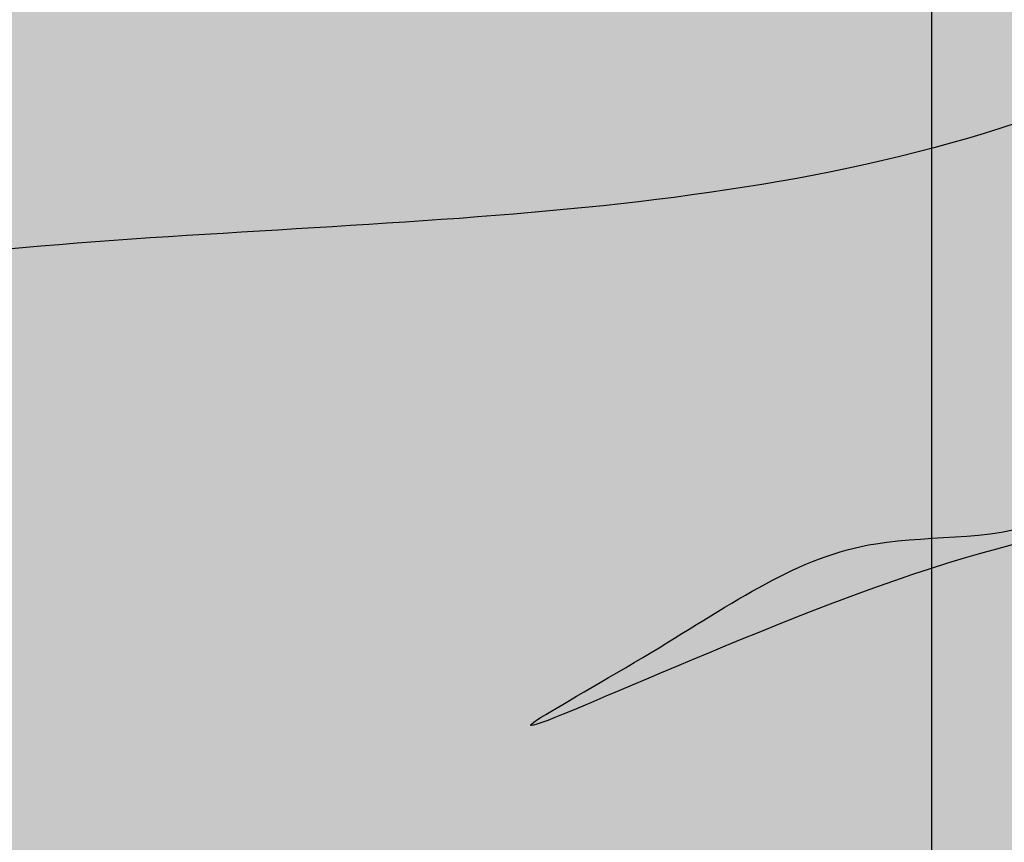
# Model space of a CAD drawing. Units: inches. Extents: x 1704 to 6393, y -157 to 1172.
# Tile 34 of 122: x 2529.29 to 2548.79, y 131.41 to 147.7. Entities that reach past the tile are written whole.
import ezdxf

# ---------------------------------------------------------------- set-up
doc = ezdxf.new("R2010")
doc.units = ezdxf.units.IN
doc.header["$MEASUREMENT"] = 0
for name, color, linetype, lineweight in [('A-ANNO-DIMS', 7, 'Continuous', 13), ('A-FURN', 8, 'Continuous', 18), ('estofado', 7, 'Continuous', 25)]:
    doc.layers.add(name, color=color, linetype=linetype, lineweight=lineweight)
doc.layers.add('A-FLOR-PATT', color=7, linetype='Continuous', lineweight=13, true_color=0xf2f2f2)
doc.styles.get("Standard").update_dxf_attribs({"font": 'arial.ttf'})
doc.dimstyles.get("Standard").update_dxf_attribs({"dimtxt": 6, "dimasz": 2, "dimexe": 0.18, "dimexo": 0.0625, "dimgap": 0.09, "dimtad": 0, "dimtih": 1, "dimtoh": 1, "dimdec": 1, "dimzin": 0, "dimdsep": 46, "dimlunit": 3, "dimtxsty": 'Standard', "dimblk": 'ARCHTICK', "dimcen": 0.09, "dimadec": 0, "dimazin": 0, "dimtfac": 1, "dimtdec": 1, "dimtofl": 0, "dimtmove": 0, "dimatfit": 3, "dimfxl": 1, "dimtolj": 1, "dimtzin": 0, "dimarcsym": 0})

# ---------------------------------------------------------------- blocks, each defined once
blk = doc.blocks.new('Cama Box Regencia LOLA')
at = {"layer": 'estofado', "ltscale": 0.2}
h = blk.add_hatch(color=256, dxfattribs=at)
h.dxf.hatch_style = 1
h.set_gradient(color1=(240, 232, 219), color2=(213, 190, 154), one_color=1, tint=0.7200000286102295, name='CURVED')
edge = h.paths.add_edge_path()
edge.add_spline(control_points=[(0.343533776195045, -0.8455058148597345), (0.2879313990920309, -0.8167160606696484), (0.2054770794474052, -0.7744470032542381), (0.0954193394759386, -0.7742416952675626), (-0.0885363502328574, -0.7276964167006668), (0.2428192566063672, -0.7672518992321216), (0.345087521536243, -0.8076697826234067), (0.3825206986321063, -0.8228555492498799)], knot_values=[0.0056315103357428, 0.0056315103357428, 0.0056315103357428, 0.0056315103357428, 0.1860138916206105, 0.2660015162584448, 0.3570871810327863, 0.5963901805690979, 0.739731738908988, 0.739731738908988, 0.739731738908988, 0.739731738908988], degree=3, periodic=0)
edge.add_spline(control_points=[(0.3825206986325611, -0.8228555492497662), (0.3974221570828149, -0.8135511441712424), (0.4121061736600496, -0.8037181558521524), (0.4266849906532571, -0.7937075488799225)], knot_values=[1.358237767273279, 1.358237767273279, 1.358237767273279, 1.358237767273279, 1.409915662372559, 1.409915662372559, 1.409915662372559, 1.409915662372559], degree=3, periodic=0)
edge.add_spline(control_points=[(0.4266849905698109, -0.7937075489369932), (0.3998777739682282, -0.7821381809783361), (0.3476761897024971, -0.7634757898491671), (0.2670618099601825, -0.7565375622627358), (0.0835725072796549, -0.7192994417154637), (0.288524529784695, -0.7446405493717521), (0.4247448861246994, -0.7759943071475277), (0.4449816270193879, -0.7810438091316882)], knot_values=[0.1043639306803623, 0.1043639306803623, 0.1043639306803623, 0.1043639306803623, 0.1896363068641149, 0.2696239315019491, 0.3607095962762907, 0.6000125958126024, 0.6446217338078729, 0.6446217338078729, 0.6446217338078729, 0.6446217338078729], degree=3, periodic=0)
edge.add_spline(control_points=[(0.4449816270197289, -0.7810438091316882), (0.5029779388527232, -0.7406836481117695), (0.5966687145296419, -0.6736247633211292), (0.7071737530245628, -0.6656573253703187), (0.7517012483331201, -0.6672238302253392)], knot_values=[1.43159032281798, 1.43159032281798, 1.43159032281798, 1.43159032281798, 1.63814180148235, 1.770695287284994, 1.770695287284994, 1.770695287284994, 1.770695287284994], degree=3, periodic=0)
edge.add_arc((0.7481853615017826, -0.767162003811734), 0.0999999999999888, 58.7920033978138, 87.98512997550938, ccw=False)
edge.add_line((0.8000000000000682, -0.6816328085782289), (0.8000000000000682, -0.154802362840428))
edge.add_line((0.8000000000000682, -0.154802362840428), (-0.7999999999999546, -0.154802362840428))
edge.add_line((-0.7999999999999546, -0.154802362840428), (-0.8000000000000682, -0.7409839258539819))
edge.add_spline(control_points=[(-0.799999999999841, -0.7409839258539251), (-0.7846451382113174, -0.74846387981205), (-0.7568940913494089, -0.7651582159765554), (-0.7559936909002545, -0.8096905380045313), (-0.7049413305308008, -0.8142555457367848), (-0.7013836936888538, -0.8139988647640733)], knot_values=[0.0122267587020837, 0.0122267587020837, 0.0122267587020837, 0.0122267587020837, 0.0594720782072034, 0.1062176618094138, 0.134458043575382, 0.134458043575382, 0.134458043575382, 0.134458043575382], degree=3, periodic=0)
edge.add_spline(control_points=[(-0.7013836936890812, -0.8139988647637892), (-0.6428309483887916, -0.8132695376718857), (-0.532520673001045, -0.8118955240036598), (-0.2390712668254764, -0.6717984706609172), (-0.3892411364554391, -0.7557901092520752), (-0.4591093260188473, -0.8070101468627512), (-0.5571511178645779, -0.795652750469742), (-0.608497950975675, -0.8409486634728295), (-0.6632498050151981, -0.8266781836207997), (-0.6991149398675134, -0.8254126024436914), (-0.719552182989446, -0.8246914287938125)], knot_values=[0, 0, 0, 0, 0.2187005959148062, 0.4120203559900679, 0.4786136596093368, 0.6046444033330721, 0.6969970394608519, 0.7456449795902803, 0.7925683322559657, 0.8547274388453192, 0.8547274388453192, 0.8547274388453192, 0.8547274388453192], degree=3, periodic=0)
edge.add_spline(control_points=[(-0.7195521829781911, -0.824691428792164), (-0.7293124663336812, -0.8248308281530967), (-0.7545977292818407, -0.8216412233076653), (-0.7742556984202338, -0.794819860189591), (-0.7939222919129634, -0.7820064600295497), (-0.799999999999841, -0.7800193173443404)], knot_values=[0.1564883932805935, 0.1564883932805935, 0.1564883932805935, 0.1564883932805935, 0.184397548386913, 0.2313764834161266, 0.2505984550882281, 0.2505984550882281, 0.2505984550882281, 0.2505984550882281], degree=3, periodic=0)
edge.add_line((-0.8000000000000682, -0.7800193173444541), (-0.7999999999999546, -0.8218505664627286))
edge.add_spline(control_points=[(-0.7999999999999546, -0.8218505664625013), (-0.7938082505512511, -0.8290217081292894), (-0.7673857405620766, -0.8512914803976059), (-0.7619109683460011, -0.8661369353891359), (-0.6555700939965164, -0.8510070218793543), (-0.7139793977868294, -0.8637526923380391), (-0.7379026254519659, -0.8623504601624176), (-0.7688129786438367, -0.8813042143888196), (-0.7854260296310259, -0.8561610219318254), (-0.7961930533253962, -0.8566031243811949), (-0.7999999999999546, -0.8573491405791173)], knot_values=[0.0595743221876141, 0.0595743221876141, 0.0595743221876141, 0.0595743221876141, 0.08075289116965, 0.1037414994169835, 0.1697200936249022, 0.1760361327243865, 0.2071371586311508, 0.2404744334261798, 0.2623408547027293, 0.2736604507987723, 0.2736604507987723, 0.2736604507987723, 0.2736604507987723], degree=3, periodic=0)
edge.add_line((-0.7999999999999546, -0.8573491405791173), (-0.8000000000000682, -0.9113562424721521))
edge.add_spline(control_points=[(-0.8000000000000682, -0.9113562424720385), (-0.7937204054647964, -0.9077594990848183), (-0.7710343135782978, -0.8978798065321029), (-0.7213062468074442, -0.9144666877443228), (-0.6268586829058905, -0.862430497409548), (-0.6896594748232019, -0.9045634991654196), (-0.7483442493064559, -0.9189273406958591), (-0.7835301183422417, -0.922920432793262), (-0.7896301351460125, -0.9477657000142585), (-0.7975786973822779, -0.955260590410262), (-0.8000000000001818, -0.9571831923294098)], knot_values=[0.0138560263374175, 0.0138560263374175, 0.0138560263374175, 0.0138560263374175, 0.0348737775836104, 0.0888666909546002, 0.1078792274429341, 0.1267378491223226, 0.1587140219647659, 0.1937574699451985, 0.2174867851300671, 0.2267221218327879, 0.2267221218327879, 0.2267221218327879, 0.2267221218327879], degree=3, periodic=0)
edge.add_line((-0.7999999999999546, -0.957183192329296), (-0.7999999999999546, -1.145824641594742))
edge.add_spline(control_points=[(-0.8000000000002955, -1.145824641594913), (-0.7271039467997298, -1.094596787649038), (-0.4885706936571524, -0.9465888221489535), (-0.0701640902225336, -0.9707493165000187), (0.237911901821235, -0.902164522332157), (0.3435337762145991, -0.845505814843193)], knot_values=[0.1168958193629841, 0.1168958193629841, 0.1168958193629841, 0.1168958193629841, 0.3797203297758731, 0.9577018633805092, 1.31379338443587, 1.31379338443587, 1.31379338443587, 1.31379338443587], degree=3, periodic=0)
h.paths.add_polyline_path([(-0.6766340706021765, -0.6101327540145576, -0.3575266660906883), (-0.7312746368313583, -0.6354535276154252, -0.3575266660894137), (-0.7059538632299791, -0.5808129613865844, -0.1647847126465284), (-0.7059538632300928, -0.2676124402649407, -0.3575266660890756), (-0.7312746368312446, -0.2129718740360431, -0.3575266660908716), (-0.6766340706020629, -0.2382926476369676, -0.0925607043966334), (-0.1295169377724505, -0.2382926476369107, -0.3575266660898965), (-0.0748763715433825, -0.2129718740360431, -0.3575266660894428), (-0.1001971451446479, -0.2676124402649407, -0.1647847126465285), (-0.1001971451445343, -0.5808129613865844, -0.3575266660890756), (-0.0748763715433825, -0.6354535276154821, -0.3575266660898962), (-0.1295169377724505, -0.6101327540146145, -0.0925607043966531)], flags=16)
h.paths.add_polyline_path([(0.0748763715433825, -0.6354535276157094, -0.3575266660910266), (0.1001971451446479, -0.5808129613865844, -0.1647847126465284), (0.1001971451445343, -0.2676124402649407, -0.3575266660890757), (0.0748763715433825, -0.2129718740360431, -0.3575266660898962), (0.1295169377724505, -0.2382926476369107, -0.0925607043966334), (0.6766340706020629, -0.2382926476369676, -0.3575266660908718), (0.7312746368312446, -0.2129718740360431, -0.3575266660894425), (0.7059538632299791, -0.2676124402649407, -0.1647847126465283), (0.7059538632300928, -0.5808129613865844, -0.3575266660890756), (0.7312746368312446, -0.6354535276154821, -0.3575266660908716), (0.6766340706020629, -0.6101327540145576, -0.0925607043966335), (0.1295169377724505, -0.6101327540146145, -0.3575266660906303)], flags=16)
h = blk.add_hatch(color=256, dxfattribs=at)
h.dxf.hatch_style = 1
h.set_gradient(color1=(206, 178, 131), color2=(227, 212, 186), one_color=1, tint=0.8100000023841857, name='CYLINDER')
edge = h.paths.add_edge_path()
edge.add_arc((0.7481853614966667, -0.7671620038115634), 0.0999999999999888, 342.0511336145294, 447.9851299725766)
edge.add_spline(control_points=[(0.7517012483331201, -0.6672238302253392), (0.7071737530245628, -0.6656573253703187), (0.5966687145298692, -0.6736247633211292), (0.5029779388527232, -0.7406836481117125), (0.4449816270195015, -0.7810438091316314)], knot_values=[1.431590322817835, 1.431590322817835, 1.431590322817835, 1.431590322817835, 1.564143808620479, 1.770695287284994, 1.770695287284994, 1.770695287284994, 1.770695287284994], degree=3, periodic=0)
edge.add_spline(control_points=[(0.4449816270195015, -0.7810438091316314), (0.4388957332065502, -0.7852790380018178), (0.4327996148541616, -0.7895089160493285), (0.4266849906533708, -0.7937075488798087)], knot_values=[1.409915662372814, 1.409915662372814, 1.409915662372814, 1.409915662372814, 1.431590322817835, 1.431590322817835, 1.431590322817835, 1.431590322817835], degree=3, periodic=0)
edge.add_spline(control_points=[(0.4266849906533708, -0.7937075488798087), (0.4121061736600496, -0.8037181558521524), (0.3974221570825875, -0.8135511441712991), (0.38252069863222, -0.8228555492498799)], knot_values=[1.358237767273037, 1.358237767273037, 1.358237767273037, 1.358237767273037, 1.409915662372815, 1.409915662372815, 1.409915662372815, 1.409915662372815], degree=3, periodic=0)
edge.add_line((0.3825206986330158, -0.8228555492493114), (0.343533776286904, -0.8455058148063584))
edge.add_spline(control_points=[(0.3435337761924302, -0.8455058148550165), (0.2379119018048641, -0.902164522335795), (-0.0701640902311738, -0.9707493164995071), (-0.4885706936571524, -0.9465888221488967), (-0.7271039467997298, -1.094596787649038), (-0.8000000000000682, -1.145824641594742)], knot_values=[0.1168958193630798, 0.1168958193630798, 0.1168958193630798, 0.1168958193630798, 0.472987340393773, 1.050968873998409, 1.313793384411202, 1.313793384411202, 1.313793384411202, 1.313793384411202], degree=3, periodic=0)
edge.add_spline(control_points=[(-0.8000000000000682, -1.145824641594742), (-0.8038896190357718, -1.14855807951244), (-0.8077744942224853, -1.151305646504738), (-0.8116551946761774, -1.154065647517199)], knot_values=[0.1028719158199011, 0.1028719158199011, 0.1028719158199011, 0.1028719158199011, 0.1168958193630799, 0.1168958193630799, 0.1168958193630799, 0.1168958193630799], degree=3, periodic=0)
edge.add_arc((-0.7536973518524519, -1.235557294053705), 0.1000000000000352, 125.4208969883762, 169.6981795679068)
edge.add_spline(control_points=[(-0.852085287466366, -1.217673946333093), (-0.8521399740518518, -1.217974812833915), (-0.8565649010855622, -1.242328483616745), (-0.8662697220019026, -1.297321141147904), (-0.8487158298532904, -1.34896742172242), (-0.8348745804664758, -1.381844109035796)], knot_values=[0.3128349436863077, 0.3128349436863077, 0.3128349436863077, 0.3128349436863077, 0.3137509534211996, 0.386958004641742, 0.4759027329026081, 0.4759027329026081, 0.4759027329026081, 0.4759027329026081], degree=3, periodic=0)
edge.add_spline(control_points=[(-0.8348745804664758, -1.38184410903591), (-0.8226532004149476, -1.367823298399059), (-0.8056354908857201, -1.352141651537124), (-0.7460155199962628, -1.32170802000337)], knot_values=[0.0062456970656236, 0.0062456970656236, 0.0062456970656236, 0.0062456970656236, 0.0554759259147193, 0.0554759259147193, 0.0554759259147193, 0.0554759259147193], degree=3, periodic=0)
edge.add_spline(control_points=[(-0.7460155200169539, -1.321708019985464), (-0.6188339616464873, -1.25080943574278), (-0.3488365122128698, -1.179158668568902), (0.0338148848931041, -1.279726484458706), (0.3977250465933366, -1.412092721352792), (0.6449024721503065, -1.106270719748692), (0.7873766543807506, -1.256744909425322), (0.8547271521993025, -1.327877176513538)], knot_values=[0.0991852523588446, 0.0991852523588446, 0.0991852523588446, 0.0991852523588446, 0.5236467270390676, 0.9270872950244264, 1.289918234564769, 1.564439021262726, 1.810554634340498, 1.810554634340498, 1.810554634340498, 1.810554634340498], degree=3, periodic=0)
edge.add_arc((0.5509678495186563, -1.223443291813453), 0.3212104454069235, 341.0267878798241, 383.7782184284114)
edge.add_arc((1.292676354991499, -0.9435407756057543), 0.4723459732861395, 162.0511336103901, 198.5657216587827, ccw=False)
h = blk.add_hatch(color=256, dxfattribs=at)
h.dxf.hatch_style = 1
h.set_gradient(color1=(240, 232, 219), color2=(137, 106, 57), one_color=1, tint=0.3799999952316284, name='CURVED')
edge = h.paths.add_edge_path()
edge.add_spline(control_points=[(-0.719552182989446, -0.8246914287938125), (-0.6991149398675134, -0.8254126024436914), (-0.6632498050151981, -0.8266781836207997), (-0.608497950975675, -0.8409486634728295), (-0.5571511178645779, -0.795652750469742), (-0.4591093260188473, -0.8070101468627512), (-0.3892411364554391, -0.7557901092520752), (-0.2390712668254764, -0.6717984706609172), (-0.532520673001045, -0.8118955240036598), (-0.6428309483887916, -0.8132695376718857), (-0.7013836936890812, -0.8139988647637892)], knot_values=[0, 0, 0, 0, 0.0621591065893537, 0.1090824592550391, 0.1577303993844675, 0.2500830355122473, 0.3761137792359825, 0.4427070828552515, 0.6360268429305131, 0.8547274388453192, 0.8547274388453192, 0.8547274388453192, 0.8547274388453192], degree=3, periodic=0)
edge.add_spline(control_points=[(-0.7013836936888538, -0.8139988647640733), (-0.7049413305308008, -0.8142555457367848), (-0.7559936909002545, -0.8096905380045313), (-0.7568940913494089, -0.7651582159765554), (-0.7846451382113174, -0.74846387981205), (-0.799999999999841, -0.7409839258539251)], knot_values=[0.0122267587020837, 0.0122267587020837, 0.0122267587020837, 0.0122267587020837, 0.0404671404680519, 0.0872127240702623, 0.134458043575382, 0.134458043575382, 0.134458043575382, 0.134458043575382], degree=3, periodic=0)
edge.add_spline(control_points=[(-0.799999999999841, -0.7409839258539251), (-0.798936373489596, -0.7431699116222604), (-0.7963938877088595, -0.7483952775559715), (-0.7912681985083055, -0.7566015403456845), (-0.7969680334608711, -0.7644035258254576), (-0.7929439183725436, -0.7707329795046576), (-0.7956241855360986, -0.7766169698310819), (-0.7985416092056994, -0.7788853679199974), (-0.7999999999999546, -0.7800193173443404)], knot_values=[0, 0, 0, 0, 0.0074537386837761, 0.0178173676883516, 0.0254983798788123, 0.0318742865004307, 0.0374248570653501, 0.0429729849735991, 0.0429729849735991, 0.0429729849735991, 0.0429729849735991], degree=3, periodic=0)
edge.add_spline(control_points=[(-0.799999999999841, -0.7800193173443404), (-0.7939222919129634, -0.7820064600295497), (-0.7742556984202338, -0.794819860189591), (-0.7545977292818407, -0.8216412233076653), (-0.7293124663336812, -0.8248308281530967), (-0.7195521829781911, -0.824691428792164)], knot_values=[0.1564883932805935, 0.1564883932805935, 0.1564883932805935, 0.1564883932805935, 0.175710364952695, 0.2226892999819086, 0.2505984550882281, 0.2505984550882281, 0.2505984550882281, 0.2505984550882281], degree=3, periodic=0)
h = blk.add_hatch(color=256, dxfattribs=at)
h.dxf.hatch_style = 1
h.set_gradient(color1=(240, 232, 219), color2=(137, 106, 57), one_color=1, tint=0.3799999952316284, name='CURVED')
edge = h.paths.add_edge_path()
edge.add_spline(control_points=[(0.3825206986321063, -0.8228555492498799), (0.345087521536243, -0.8076697826234067), (0.2428192566063672, -0.7672518992321216), (-0.0885363502328574, -0.7276964167006668), (0.0954193394759386, -0.7742416952675626), (0.2054770794474052, -0.7744470032542381), (0.2879313990920309, -0.8167160606696484), (0.343533776195045, -0.8455058148597345)], knot_values=[0.0056315103357428, 0.0056315103357428, 0.0056315103357428, 0.0056315103357428, 0.1489730686756328, 0.3882760682119444, 0.479361732986286, 0.5593493576241202, 0.739731738908988, 0.739731738908988, 0.739731738908988, 0.739731738908988], degree=3, periodic=0)
edge.add_line((0.343533776195045, -0.8455058148597913), (0.3825206986321063, -0.8228555492498799))
for points, knots in [([(-0.7013836936890812, -0.8139988647637892), (-0.6428309483887775, -0.8132695376718778), (-0.5325206730010296, -0.8118955240036225), (-0.2390712668254173, -0.6717984706608711), (-0.3892411364555083, -0.755790109252117), (-0.4591093260187714, -0.8070101468627889), (-0.5571511178644899, -0.795652750469717), (-0.6084979509757439, -0.8409486634728317), (-0.6632498050152652, -0.8266781836208043), (-0.6991149398675783, -0.8254126024437319), (-0.719552182989446, -0.8246914287938125)], [0, 0, 0, 0, 0.2187005959148062, 0.4120203559900679, 0.4786136596093368, 0.6046444033330721, 0.6969970394608519, 0.7456449795902803, 0.7925683322559657, 0.8547274388453192, 0.8547274388453192, 0.8547274388453192, 0.8547274388453192]), ([(-0.8116551946761774, -1.154065647517199), (-0.7350455857787211, -1.099579968801037), (-0.493473113061782, -0.9463057365681493), (-0.0701640902311738, -0.9707493164995071), (0.2379119018048641, -0.902164522335795), (0.3435337761924302, -0.8455058148550165)], [0.1028719158199011, 0.1028719158199011, 0.1028719158199011, 0.1028719158199011, 0.3797203297758731, 0.9577018633805092, 1.313793384411202, 1.313793384411202, 1.313793384411202, 1.313793384411202])]:
    blk.add_open_spline(points, degree=3, knots=knots, dxfattribs=at)
blk = doc.blocks.new('_ArchTick')
at = {"color": 0, "linetype": 'ByBlock', "const_width": 0.15}
blk.add_lwpolyline([(-0.5, -0.5), (0.5, 0.5)], dxfattribs=at)
blk = doc.blocks.new('*D93')
at = {"layer": 'A-ANNO-DIMS', "color": 0, "lineweight": -2, "transparency": 16777216}
for p, q in [((2605.286074000001, 895.2129740000005), (1829.697551000002, 895.2129740000003)), ((1829.877551000002, 895.2129740000003), (1829.877551000002, 495.8664119263302)), ((1829.877551000002, 90.2129739999999), (1829.877551000002, 489.5595360736699)), ((2605.286074000001, 90.21297400000003), (1829.697551000002, 90.2129739999999))]:
    blk.add_line(p, q, dxfattribs=at)
at = {"layer": 'Defpoints', "color": 0, "lineweight": -3, "transparency": 16777216}
for p in [(2605.348574000001, 895.2129740000005), (1829.877551000002, 90.2129739999999), (2605.348574000001, 90.21297400000003)]:
    blk.add_point(p, dxfattribs=at)
at = {"layer": 'A-ANNO-DIMS', "color": 0, "lineweight": -2, "transparency": 16777216, "xscale": 2, "yscale": 2, "zscale": 2}
for p, rotation in [((1829.877551000002, 895.2129740000003), 90), ((1829.877551000002, 90.2129739999999), 270)]:
    blk.add_blockref('_ArchTick', p, dxfattribs=dict(at, rotation=rotation))
at = {"layer": 'A-ANNO-DIMS', "color": 0, "transparency": 16777216, "insert": (1829.877551000001, 492.7129739999994), "char_height": 6, "attachment_point": 5}
blk.add_mtext('\\A1;805', dxfattribs=at)
blk = doc.blocks.new('*D105')
at = {"layer": 'A-ANNO-DIMS', "color": 0, "lineweight": -2, "transparency": 16777216}
for p, q in [((2451.737975, 615.150474), (2451.737975, -64.9670259999999)), ((2547.348574, 615.150474), (2547.348574, -64.9670259999999)), ((2451.737975, -64.787026), (2489.908936164393, -64.787026)), ((2547.348574, -64.787026), (2509.177612835607, -64.787026))]:
    blk.add_line(p, q, dxfattribs=at)
at = {"layer": 'Defpoints', "color": 0, "lineweight": -3, "transparency": 16777216}
for p in [(2451.737975, 615.212974), (2547.348574, 615.212974), (2547.348574, -64.787026)]:
    blk.add_point(p, dxfattribs=at)
at = {"layer": 'A-ANNO-DIMS', "color": 0, "lineweight": -2, "transparency": 16777216, "xscale": 2, "yscale": 2, "zscale": 2, "rotation": 180}
blk.add_blockref('_ArchTick', (2451.737975, -64.787026), dxfattribs=at)
at = {"layer": 'A-ANNO-DIMS', "color": 0, "lineweight": -2, "transparency": 16777216, "xscale": 2, "yscale": 2, "zscale": 2}
blk.add_blockref('_ArchTick', (2547.348574, -64.787026), dxfattribs=at)
at = {"layer": 'A-ANNO-DIMS', "color": 0, "transparency": 16777216, "insert": (2499.5432745, -64.787026), "char_height": 6, "attachment_point": 5}
blk.add_mtext('\\A1;95.61', dxfattribs=at)

msp = doc.modelspace()

# ---------------------------------------------------------------- hatches: boundary and pattern name
at = {"layer": 'A-FLOR-PATT', "transparency": 33554528}
h = msp.add_hatch(color=256, dxfattribs=at)
h.dxf.hatch_style = 1
h.paths.add_polyline_path([(2325.348574056059, 863.2129735309796), (2325.348574056059, 887.2129735309796), (2263.348574056059, 887.2129735309796), (2167.348574056059, 887.2129735309794), (2081.348574056061, 887.2129735309792), (2081.348574056061, 719.2129735309785), (2277.348574056059, 719.2129735309787), (2277.348574056059, 711.2129735309788), (2277.348574056059, 372.212973530979), (2349.348574056059, 372.212973530979), (2381.348574056059, 372.2129735309789), (2381.348574056059, 364.2129735309789), (2353.348574056059, 364.2129735309789), (2353.348574056059, 270.2129735309788), (2381.348574056059, 270.2129735309788), (2381.348574056059, 266.2129735309788), (2357.348574056059, 266.2129735309788), (2357.348574056059, 98.21297353097884), (2381.348574056059, 98.21297353097897), (2385.181056550604, 98.21297353097884), (2386.482186711948, 98.21297353097884), (2424.21496140017, 98.21297353097884), (2425.516091561514, 98.21297353097884), (2429.348574056059, 98.21297353097897), (2597.348574056059, 98.21297353097884), (2597.348574056059, 146.2129735309788), (2597.348574056059, 218.2129735309788), (2597.348574056059, 266.2129735309788), (2423.348574056059, 266.2129735309788), (2423.348574056059, 270.2129735309788), (2473.348574056059, 270.2129735309788), (2473.348574056059, 294.2129735309789), (2477.348574056059, 294.2129735309789), (2477.348574056059, 270.2129735309788), (2547.348574056059, 270.2129735309788), (2547.348574056059, 364.2129735309788), (2477.348574056059, 364.2129735309788), (2477.348574056059, 318.2129735309788), (2473.348574056059, 318.2129735309787), (2473.348574056059, 364.2129735309789), (2423.348574056059, 364.2129735309788), (2423.348574056059, 372.2129735309788), (2469.348574056059, 372.2129735309788), (2469.348574056059, 459.2129735309789), (2469.348574056059, 538.2129735309788), (2350.348574056059, 538.2129735309788), (2350.348574056059, 565.7129735309788), (2358.348574056059, 565.7129735309788), (2358.348574056059, 545.2129735309788), (2420.348574056059, 545.2129735309788), (2420.348574056059, 610.2129735309788), (2358.348574056059, 610.2129735309788), (2358.348574056059, 589.7129735309788), (2350.348574056059, 589.7129735309788), (2350.348574056059, 615.2129735309788), (2425.348574056059, 615.2129735309788), (2425.348574056059, 607.2129735309788), (2425.348574056059, 546.2129735309788), (2469.348574056059, 546.2129735309788), (2514.34857405606, 546.212973530979), (2514.34857405606, 607.2129735309788), (2449.348574056059, 607.2129735309788), (2449.348574056059, 615.2129735309788), (2451.737974987759, 615.2129735309788), (2451.737974987759, 659.2129735309788), (2427.737974987759, 659.2129735309788), (2427.737974987759, 665.2129735309788), (2367.737974987758, 665.2129735309788), (2367.737974987758, 667.2129735309788), (2367.737974987758, 711.2129735309788), (2325.348574056059, 711.2129735309788), (2325.348574056059, 719.2129735309785), (2325.348574056059, 755.2129735309787), (2325.348574056059, 763.2129735309788)])
h.paths.add_polyline_path([(2233.85817000392, 822.532660166629, -0.1872470486944155), (2233.85817000392, 809.1396667958562), (2231.697030374885, 808.8044951349628, 0.0848927708004382), (2233.130501812631, 814.4858417746204), (2230.423974436808, 814.4858417746204, -0.1042581087707907), (2228.553363812687, 808.3129425443484), (2217.750790159711, 807.1555239386723, -0.2222222222222219), (2217.750790159711, 824.5168030238124), (2228.553363812687, 823.3593844181363, -0.1042581087707933), (2230.423974436808, 817.1864851878643), (2233.130501812631, 817.1864851878643, 0.08489277080044), (2231.697030374885, 822.8678318275219)], flags=16)
h.paths.add_polyline_path([(2213.621360876743, 833.1974425663823), (2213.621360876743, 798.4748843961024), (2156.047684459484, 798.4748843961034), (2156.047684459485, 833.1974425663813)], flags=16)
h.paths.add_polyline_path([(2203.931929661768, 848.0987249710489), (2205.089348267444, 837.2961513180724, -0.2222222222222264), (2187.728069182304, 837.2961513180724), (2188.88548778798, 848.0987249710485, -0.104258108770792), (2195.058387018252, 849.9693355951691), (2195.058387018252, 852.6758629709927, 0.084892770800438), (2189.377040378595, 851.2423915332469), (2189.712212039488, 853.4035311622828, -0.1872470486944166), (2203.105205410261, 853.4035311622828), (2203.440377071154, 851.2423915332469, 0.084892770800438), (2197.759030431496, 852.6758629709927), (2197.759030431496, 849.9693355951691, -0.1042581087707896)], flags=16)
h.paths.add_polyline_path([(2181.940976153924, 837.2961513180726, -0.2222222222222323), (2164.579697068783, 837.2961513180724), (2165.73711567446, 848.0987249710487, -0.1042581087707905), (2171.910014904732, 849.9693355951691), (2171.910014904732, 852.6758629709927, 0.0848927708004445), (2166.228668265074, 851.2423915332469), (2166.563839925967, 853.403531162283, -0.1872470486944096), (2179.95683329674, 853.4035311622828), (2180.292004957633, 851.2423915332465, 0.0848927708004458), (2174.610658317976, 852.6758629709927), (2174.610658317976, 849.9693355951691, -0.104258108770801), (2180.783557548248, 848.0987249710482)], flags=16)
h.paths.add_polyline_path([(2205.089348267444, 794.376175644412), (2203.931929661768, 783.5736019914364, -0.1042581087707934), (2197.759030431496, 781.7029913673155), (2197.759030431496, 778.9964639914921, 0.084892770800439), (2203.440377071154, 780.4299354292382), (2203.105205410261, 778.2687958002022, -0.1872470486944172), (2189.712212039488, 778.2687958002018), (2189.377040378595, 780.4299354292377, 0.0848927708004369), (2195.058387018252, 778.9964639914919), (2195.058387018252, 781.7029913673153, -0.1042581087707904), (2188.88548778798, 783.5736019914358), (2187.728069182304, 794.3761756444126, -0.2222222222222231)], flags=16)
h.paths.add_polyline_path([(2181.940976153924, 794.376175644412), (2180.783557548248, 783.5736019914364, -0.1042581087708008), (2174.610658317976, 781.7029913673153), (2174.610658317976, 778.9964639914921, 0.0848927708004458), (2180.292004957633, 780.4299354292382), (2179.95683329674, 778.268795800202, -0.1872470486944096), (2166.563839925967, 778.2687958002018), (2166.228668265074, 780.4299354292378, 0.0848927708004446), (2171.910014904732, 778.9964639914919), (2171.910014904732, 781.7029913673153, -0.1042581087707904), (2165.73711567446, 783.5736019914358), (2164.579697068783, 794.3761756444123, -0.2222222222222294)], flags=16)
h.paths.add_polyline_path([(2151.918255176517, 807.1555239386723), (2141.115681523541, 808.3129425443484, -0.1042581087707911), (2139.24507089942, 814.4858417746204), (2136.538543523597, 814.4858417746204, 0.08489277080044), (2137.972014961343, 808.8044951349626), (2135.810875332307, 809.1396667958562, -0.1872470486944109), (2135.810875332307, 822.5326601666285), (2137.972014961343, 822.8678318275221, 0.0848927708004416), (2136.538543523597, 817.1864851878643), (2139.24507089942, 817.1864851878643, -0.104258108770793), (2141.115681523541, 823.3593844181363), (2151.918255176517, 824.5168030238124, -0.2222222222222205)], flags=16)
h.paths.add_polyline_path([(2357.868011454448, 363.4102250290031), (2358.813881560335, 363.4102250290031, 0.7537604849588476)], flags=16)
h.paths.add_polyline_path([(2372.241054283868, 363.1167008961685), (2372.248110816919, 363.1167008961685), (2372.248110816919, 363.3425764997267), (2371.30224071103, 363.3425764997267), (2371.30224071103, 363.1392706554335, -1.360391292333951)], flags=16)
h.paths.add_polyline_path([(2371.309297244092, 272.7157694655011), (2371.30224071103, 272.7157694655011), (2371.30224071103, 272.4898938619428), (2372.248110816919, 272.4898938619428), (2372.248110816919, 272.6931997062759, -1.360391292393621)], flags=16)
h.paths.add_polyline_path([(2357.875067987504, 272.7157694655011), (2357.868011454452, 272.7157694655011), (2357.868011454452, 272.4898938619428), (2358.813881560341, 272.4898938619428), (2358.813881560341, 272.6931997062361, -1.360391292333948)], flags=16)
h.paths.add_polyline_path([(2353.768696905258, 363.0736921025416), (2376.347425366111, 363.0736921025416), (2376.347425366111, 272.7587782591281), (2353.768696905258, 272.7587782591281)], flags=16)
h.paths.add_polyline_path([(2354.772195947961, 362.0701930598379), (2375.343926323407, 362.0701930598379), (2375.343926323407, 273.7622773018316), (2354.772195947961, 273.7622773018318)], flags=0)
h.paths.add_polyline_path([(2357.868011454452, 363.3425764997267), (2358.813881560341, 363.3425764997266), (2358.813881560341, 363.1167008961684), (2357.868011454452, 363.1167008961684)], flags=16)
h.paths.add_polyline_path([(2359.287941640134, 359.1843485433627), (2359.287941640134, 360.0631949744305), (2370.828180631237, 360.0631949744362), (2370.828180631237, 359.1843485433769), (2374.332057422314, 359.1843485433812), (2374.332057422312, 358.4635369582513), (2372.835178716611, 358.4635369582524), (2372.835178716611, 357.5410357047662), (2374.332057422314, 357.5410357047678), (2374.332057422312, 356.8202241196381), (2372.835178716611, 356.820224119639), (2372.835178716611, 355.897722866153), (2374.332057422314, 355.8977228661546), (2374.332057422312, 355.1769112810248), (2372.835178716611, 355.1769112810259), (2372.835178716611, 354.2544100275397), (2374.332057422334, 354.2544100275415), (2374.332057422331, 353.5335984424117), (2372.835178716631, 353.5335984424126), (2372.835178716631, 352.6110971889265), (2374.332057422334, 352.6110971889282), (2374.332057422331, 351.8902856037984), (2372.835178716631, 351.8902856037993), (2372.835178716631, 350.9677843503132), (2374.332057422334, 350.967784350315), (2374.332057422331, 350.2469727651852), (2372.835178716631, 350.2469727651861), (2372.835178716631, 349.3244715117), (2374.332057422334, 349.3244715117017), (2374.332057422331, 348.603659926572), (2372.835178716631, 348.6036599265729), (2372.835178716631, 347.6811586730868), (2374.332057422334, 347.6811586730886), (2374.332057422331, 346.9603470879587), (2372.835178716631, 346.9603470879598), (2372.835178716631, 346.0378458344735), (2374.332057422334, 346.0378458344753), (2374.332057422331, 345.3170342493456), (2372.835178716631, 345.3170342493465), (2372.835178716631, 344.3945329958605), (2374.332057422334, 344.3945329958621), (2374.332057422331, 343.6737214107324), (2372.835178716631, 343.6737214107334), (2372.835178716631, 342.751220157247), (2374.332057422334, 342.7512201572489), (2374.332057422331, 342.0304085721191), (2372.835178716631, 342.03040857212), (2372.835178716631, 341.1079073186338), (2374.332057422334, 341.1079073186356), (2374.332057422331, 340.3870957335057), (2372.835178716631, 340.3870957335066), (2372.835178716631, 339.4645944800207), (2374.332057422334, 339.4645944800223), (2374.332057422331, 338.7437828948924), (2372.835178716648, 338.7437828948933), (2372.835178716648, 337.8212816414076), (2374.332057422334, 337.8212816414093), (2374.332057422331, 337.1004700562794), (2372.835178716648, 337.1004700562803), (2372.835178716648, 336.1779688027942), (2374.332057422334, 336.1779688027961), (2374.332057422331, 335.4571572176662), (2372.835178716648, 335.4571572176673), (2372.835178716648, 334.5346559641809), (2374.332057422334, 334.5346559641828), (2374.332057422331, 333.8138443790529), (2372.835178716648, 333.8138443790539), (2372.835178716648, 332.8913431255679), (2374.332057422334, 332.8913431255696), (2374.332057422331, 332.1705315404397), (2372.835178716648, 332.1705315404406), (2372.835178716648, 331.2480302869545), (2374.332057422334, 331.2480302869563), (2374.332057422331, 330.5272187018265), (2372.835178716648, 330.5272187018273), (2372.835178716648, 329.6047174483413), (2374.332057422334, 329.6047174483431), (2374.332057422331, 328.8839058632133), (2372.835178716648, 328.8839058632143), (2372.835178716648, 327.9614046097282), (2374.332057422334, 327.9614046097298), (2374.332057422331, 327.2405930246), (2372.835178716648, 327.2405930246009), (2372.835178716648, 326.3180917711149), (2374.332057422334, 326.3180917711167), (2374.332057422331, 325.5972801859869), (2372.835178716648, 325.5972801859877), (2372.835178716648, 324.6747789325016), (2374.332057422334, 324.6747789325034), (2374.332057422331, 323.9539673473736), (2372.835178716648, 323.9539673473746), (2372.835178716648, 323.0314660938884), (2374.332057422334, 323.0314660938901), (2374.332057422331, 322.3106545087603), (2372.835178716648, 322.3106545087613), (2372.835178716648, 321.3881532552753), (2374.332057422334, 321.388153255277), (2374.332057422331, 320.6673416701471), (2372.835178716648, 320.6673416701481), (2372.835178716648, 319.7448404166621), (2374.332057422334, 319.7448404166638), (2374.332057422331, 319.0240288315339), (2372.835178716648, 319.0240288315348), (2372.835178716648, 318.1015275780487), (2374.332057422334, 318.1015275780504), (2374.332057422331, 317.3807159929205), (2372.835178716648, 317.3807159929214), (2372.835178716648, 316.4582147394357), (2374.332057422334, 316.4582147394373), (2374.332057422331, 315.7374031543073), (2372.835178716648, 315.7374031543084), (2372.835178716648, 314.8149019008223), (2374.332057422334, 314.8149019008241), (2374.332057422331, 314.0940903156943), (2372.835178716648, 314.0940903156952), (2372.835178716648, 313.171589062209), (2374.332057422334, 313.1715890622108), (2374.332057422331, 312.450777477081), (2372.835178716648, 312.4507774770819), (2372.835178716648, 311.5282762235959), (2374.332057422334, 311.5282762235977), (2374.332057422331, 310.8074646384678), (2372.835178716648, 310.8074646384687), (2372.835178716648, 309.8849633849827), (2374.332057422334, 309.8849633849844), (2374.332057422331, 309.1641517998546), (2372.835178716648, 309.1641517998555), (2372.835178716648, 308.2416505463693), (2374.332057422334, 308.2416505463712), (2374.332057422331, 307.5208389612412), (2372.835178716648, 307.5208389612421), (2372.835178716648, 306.5983377077562), (2374.332057422334, 306.598337707758), (2374.332057422331, 305.8775261226281), (2372.835178716648, 305.8775261226289), (2372.835178716648, 304.955024869143), (2374.332057422334, 304.9550248691447), (2374.332057422331, 304.2342132840149), (2372.835178716648, 304.2342132840158), (2372.835178716648, 303.3117120305298), (2374.332057422334, 303.3117120305316), (2374.332057422331, 302.5909004454018), (2372.835178716648, 302.5909004454027), (2372.835178716648, 301.6683991919165), (2374.332057422334, 301.6683991919183), (2374.332057422331, 300.9475876067885), (2372.835178716648, 300.9475876067894), (2372.835178716648, 300.0250863533033), (2374.332057422334, 300.025086353305), (2374.332057422331, 299.3042747681752), (2372.835178716648, 299.3042747681761), (2372.835178716648, 298.3817735146902), (2374.332057422334, 298.3817735146919), (2374.332057422331, 297.6609619295621), (2372.835178716648, 297.6609619295629), (2372.835178716648, 296.7384606760769), (2374.332057422334, 296.7384606760786), (2374.332057422331, 296.0176490909488), (2372.835178716648, 296.0176490909498), (2372.835178716648, 295.0951478374636), (2374.332057422334, 295.0951478374653), (2374.332057422331, 294.3743362523355), (2372.835178716648, 294.3743362523364), (2372.835178716648, 293.4518349988504), (2374.332057422334, 293.4518349988522), (2374.332057422331, 292.7310234137224), (2372.835178716648, 292.7310234137233), (2372.835178716648, 291.8085221602371), (2374.332057422334, 291.8085221602389), (2374.332057422331, 291.0877105751091), (2372.835178716648, 291.08771057511), (2372.835178716648, 290.165209321624), (2374.332057422334, 290.1652093216256), (2374.332057422331, 289.4443977364957), (2372.835178716648, 289.4443977364966), (2372.835178716648, 288.5218964830108), (2374.332057422334, 288.5218964830125), (2374.332057422331, 287.8010848978827), (2372.835178716648, 287.8010848978836), (2372.835178716648, 286.8785836443975), (2374.332057422334, 286.8785836443993), (2374.332057422331, 286.1577720592695), (2372.835178716648, 286.1577720592703), (2372.835178716648, 285.2352708057842), (2374.332057422334, 285.2352708057861), (2374.332057422331, 284.5144592206562), (2372.835178716648, 284.514459220657), (2372.835178716648, 283.5919579671712), (2374.332057422334, 283.5919579671728), (2374.332057422331, 282.871146382043), (2372.835178716648, 282.8711463820439), (2372.835178716648, 281.9486451285579), (2374.332057422334, 281.9486451285596), (2374.332057422331, 281.2278335434298), (2372.835178716648, 281.2278335434307), (2372.835178716648, 280.3053322899446), (2374.332057422334, 280.3053322899464), (2374.332057422331, 279.5845207048164), (2372.835178716648, 279.5845207048174), (2372.835178716648, 278.6620194513314), (2374.332057422334, 278.6620194513331), (2374.332057422331, 277.9412078662033), (2372.835178716648, 277.9412078662043), (2372.835178716648, 277.0187066127184), (2374.332057422334, 277.0187066127201), (2374.332057422331, 276.29789502759), (2370.828180631244, 276.2978950275922), (2370.828180631244, 275.7692753872335), (2359.287941640128, 275.7692753872392), (2359.287941640128, 276.2978950275993), (2355.784064849037, 276.2978950276015), (2355.784064849037, 277.0187066126971), (2357.280943554723, 277.0187066126989), (2357.280943554723, 277.9412078662137), (2355.784064849037, 277.9412078662145), (2355.784064849037, 278.6620194513103), (2357.280943554723, 278.6620194513122), (2357.280943554723, 279.5845207048271), (2355.784064849037, 279.584520704828), (2355.784064849037, 280.3053322899236), (2357.280943554723, 280.3053322899253), (2357.280943554723, 281.2278335434403), (2355.784064849037, 281.2278335434412), (2355.784064849037, 281.9486451285369), (2357.280943554723, 281.9486451285387), (2357.280943554723, 282.8711463820535), (2355.784064849037, 282.8711463820543), (2355.784064849037, 283.5919579671501), (2357.280943554723, 283.591957967152), (2357.280943554723, 284.5144592206668), (2355.784064849037, 284.5144592206676), (2355.784064849037, 285.2352708057632), (2357.280943554723, 285.2352708057651), (2357.280943554723, 286.1577720592801), (2355.784064849037, 286.1577720592809), (2355.784064849037, 286.8785836443766), (2357.280943554723, 286.8785836443784), (2357.280943554723, 287.8010848978931), (2355.784064849037, 287.8010848978941), (2355.784064849037, 288.5218964829895), (2357.280943554723, 288.5218964829913), (2357.280943554723, 289.4443977365064), (2355.784064849037, 289.4443977365072), (2355.784064849037, 290.1652093216029), (2357.280943554723, 290.1652093216047), (2357.280943554723, 291.0877105751197), (2355.784064849037, 291.0877105751206), (2355.784064849037, 291.8085221602161), (2357.280943554723, 291.8085221602179), (2357.280943554723, 292.7310234137328), (2355.784064849037, 292.7310234137337), (2355.784064849037, 293.4518349988293), (2357.280943554723, 293.451834998831), (2357.280943554723, 294.3743362523461), (2355.784064849037, 294.3743362523469), (2355.784064849037, 295.0951478374426), (2357.280943554723, 295.0951478374445), (2357.280943554723, 296.0176490909594), (2355.784064849037, 296.0176490909601), (2355.784064849037, 296.7384606760557), (2357.280943554723, 296.7384606760575), (2357.280943554723, 297.6609619295724), (2355.784064849037, 297.6609619295734), (2355.784064849037, 298.3817735146691), (2357.280943554723, 298.3817735146709), (2357.280943554723, 299.3042747681858), (2355.784064849037, 299.3042747681866), (2355.784064849037, 300.0250863532823), (2357.280943554723, 300.0250863532841), (2357.280943554723, 300.9475876067989), (2355.784064849037, 300.9475876067997), (2355.784064849037, 301.6683991918954), (2357.280943554723, 301.6683991918973), (2357.280943554723, 302.5909004454123), (2355.784064849037, 302.5909004454133), (2355.784064849037, 303.3117120305088), (2357.280943554723, 303.3117120305105), (2357.280943554723, 304.2342132840254), (2355.784064849037, 304.2342132840262), (2355.784064849037, 304.9550248691219), (2357.280943554723, 304.9550248691238), (2357.280943554723, 305.8775261226386), (2355.784064849037, 305.8775261226394), (2355.784064849037, 306.5983377077352), (2357.280943554723, 306.5983377077369), (2357.280943554723, 307.5208389612518), (2355.784064849037, 307.5208389612528), (2355.784064849037, 308.2416505463484), (2357.280943554723, 308.2416505463501), (2357.280943554723, 309.1641517998652), (2355.784064849037, 309.1641517998661), (2355.784064849037, 309.8849633849617), (2357.280943554723, 309.8849633849634), (2357.280943554723, 310.8074646384782), (2355.784064849037, 310.8074646384791), (2355.784064849037, 311.5282762235748), (2357.280943554723, 311.5282762235767), (2357.280943554723, 312.4507774770916), (2355.784064849037, 312.4507774770925), (2355.784064849037, 313.171589062188), (2357.280943554723, 313.1715890621898), (2357.280943554723, 314.0940903157049), (2355.784064849037, 314.0940903157058), (2355.784064849037, 314.8149019008013), (2357.280943554723, 314.8149019008032), (2357.280943554723, 315.7374031543179), (2355.784064849037, 315.7374031543187), (2355.784064849037, 316.4582147394146), (2357.280943554723, 316.4582147394165), (2357.280943554723, 317.3807159929311), (2355.784064849037, 317.3807159929321), (2355.784064849037, 318.1015275780277), (2357.280943554723, 318.1015275780295), (2357.280943554723, 319.0240288315445), (2355.784064849037, 319.0240288315454), (2355.784064849037, 319.744840416641), (2357.280943554723, 319.7448404166428), (2357.280943554723, 320.6673416701576), (2355.784064849037, 320.6673416701585), (2355.784064849037, 321.3881532552541), (2357.280943554723, 321.388153255256), (2357.280943554723, 322.3106545087708), (2355.784064849037, 322.3106545087718), (2355.784064849037, 323.0314660938674), (2357.280943554723, 323.0314660938692), (2357.280943554723, 323.9539673473843), (2355.784064849037, 323.9539673473851), (2355.784064849037, 324.6747789324806), (2357.280943554723, 324.6747789324824), (2357.280943554723, 325.5972801859974), (2355.784064849037, 325.5972801859983), (2355.784064849037, 326.3180917710939), (2357.280943554723, 326.3180917710958), (2357.280943554723, 327.2405930246105), (2355.784064849037, 327.2405930246113), (2355.784064849037, 327.9614046097071), (2357.280943554723, 327.961404609709), (2357.280943554723, 328.8839058632238), (2355.784064849037, 328.8839058632245), (2355.784064849037, 329.6047174483202), (2357.280943554723, 329.604717448322), (2357.280943554723, 330.527218701837), (2355.784064849037, 330.5272187018379), (2355.784064849037, 331.2480302869335), (2357.280943554723, 331.2480302869353), (2357.280943554723, 332.1705315404502), (2355.784064849037, 332.170531540451), (2355.784064849037, 332.8913431255468), (2357.280943554723, 332.8913431255486), (2357.280943554723, 333.8138443790634), (2355.784064849037, 333.8138443790642), (2355.784064849037, 334.5346559641599), (2357.280943554723, 334.5346559641618), (2357.280943554723, 335.4571572176767), (2355.784064849037, 335.4571572176776), (2355.784064849037, 336.1779688027732), (2357.280943554723, 336.177968802775), (2357.280943554723, 337.1004700562898), (2355.784064849037, 337.1004700562908), (2355.784064849037, 337.8212816413864), (2357.280943554723, 337.8212816413883), (2357.280943554723, 338.7437828949031), (2355.784064849037, 338.743782894904), (2355.784064849037, 339.4645944799996), (2357.280943554706, 339.4645944800013), (2357.280943554706, 340.3870957335163), (2355.784064849037, 340.3870957335173), (2355.784064849037, 341.1079073186129), (2357.280943554706, 341.1079073186146), (2357.280943554706, 342.0304085721296), (2355.784064849037, 342.0304085721304), (2355.784064849037, 342.7512201572262), (2357.280943554706, 342.751220157228), (2357.280943554706, 343.6737214107429), (2355.784064849037, 343.6737214107437), (2355.784064849037, 344.3945329958394), (2357.280943554706, 344.3945329958412), (2357.280943554706, 345.317034249356), (2355.784064849037, 345.3170342493569), (2355.784064849037, 346.0378458344526), (2357.280943554706, 346.0378458344544), (2357.280943554706, 346.9603470879692), (2355.784064849037, 346.9603470879701), (2355.784064849037, 347.6811586730658), (2357.280943554706, 347.6811586730677), (2357.280943554706, 348.6036599265824), (2355.784064849037, 348.6036599265833), (2355.784064849037, 349.324471511679), (2357.280943554706, 349.3244715116809), (2357.280943554706, 350.2469727651956), (2355.784064849037, 350.2469727651966), (2355.784064849037, 350.9677843502922), (2357.280943554706, 350.9677843502939), (2357.280943554706, 351.8902856038089), (2355.784064849037, 351.8902856038098), (2355.784064849037, 352.6110971889055), (2357.280943554706, 352.6110971889072), (2357.280943554706, 353.5335984424222), (2355.784064849037, 353.533598442423), (2355.784064849037, 354.2544100275187), (2357.280943554686, 354.2544100275204), (2357.280943554686, 355.1769112810354), (2355.784064849017, 355.1769112810362), (2355.784064849017, 355.897722866132), (2357.280943554686, 355.8977228661338), (2357.280943554686, 356.8202241196486), (2355.784064849017, 356.8202241196495), (2355.784064849017, 357.5410357047453), (2357.280943554686, 357.5410357047471), (2357.280943554686, 358.4635369582618), (2355.784064849017, 358.4635369582626), (2355.784064849017, 359.1843485433584)], flags=0)

# ---------------------------------------------------------------- block references
at = {"layer": 'A-FURN', "xscale": 39.22313671019584, "yscale": 39.22313671019584, "zscale": 39.22313671019584, "rotation": 180}
msp.add_blockref('Cama Box Regencia LOLA', (2527.569415053021, 106.0625493409584), dxfattribs=at)

# ---------------------------------------------------------------- dimensions: what is measured, and where the dimension line sits
at = {"layer": 'A-ANNO-DIMS'}
dim = msp.add_linear_dim(base=(1829.877551000002, 90.2129739999999), p1=(2605.348574000001, 895.212974), p2=(2605.348574000001, 90.21297399999999), angle=90, dimstyle='Standard', override={"dimdec": 0, "dimlfac": 1, "dimrnd": 0, "dimzin": 0, "dimdsep": 46, "dimlunit": 2}, dxfattribs=at)
dim.commit()
dim.dimension.update_dxf_attribs({"geometry": '*D93', "text_midpoint": (1829.877551000001, 492.7129739999994)})
dim = msp.add_linear_dim(base=(2547.348574, -64.787026), p1=(2451.737975, 615.212974), p2=(2547.348574, 615.212974), dimstyle='Standard', override={"dimdec": 2, "dimlfac": 1, "dimrnd": 0, "dimzin": 0, "dimdsep": 46, "dimlunit": 2}, dxfattribs=at)
dim.commit()
dim.dimension.update_dxf_attribs({"geometry": '*D105', "text_midpoint": (2499.5432745, -64.787026)})

doc.saveas('drawing.dxf')
